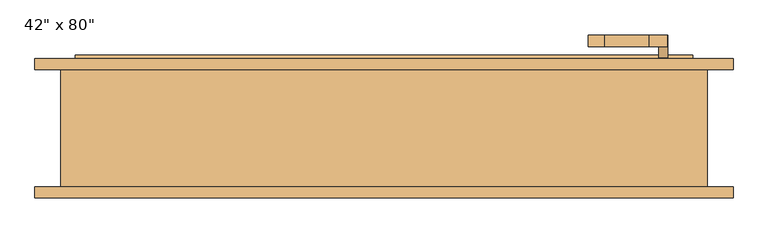
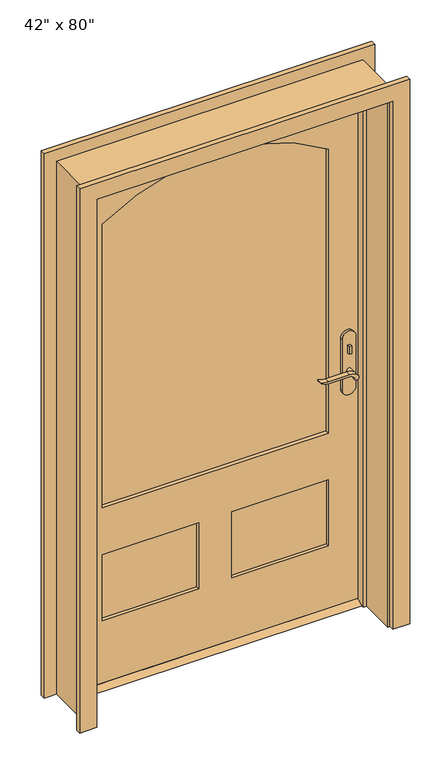
"""IFC4 building model written with IfcOpenShell, lengths in millimetres: door geometry."""

from ifc_helpers import new_model, si_unit, point, frame, frame_2d, origin, place, context, project, spatial, polyline, circle_curve, trimmed, segment, composite_curve, outline, extrude, faceted_brep, source, transform, mapped, element, save


def door_3b8e8068(model_context):
    return source(origin(), model_context, "Body", "SolidModel", [
        extrude(outline(polyline([(63.5, 12.7), (98.425, 12.7), (123.825, 0.0), (38.1, 0.0), (63.5, 12.7)])), frame((-533.4, 0.0, 0.0), z_axis=(1.0, 0.0, 0.0), x_axis=(0.0, 1.0, 0.0)), (0.0, 0.0, 1.0), 1066.8),
        extrude(outline(polyline([(487.6, 43.5), (477.6, 43.5), (477.6, 53.5), (487.6, 53.5), (487.6, 43.5)])), frame((0.0, 0.0, 981.9), z_axis=(0.0, 0.0, 1.0), x_axis=(1.0, 0.0, 0.0)), (0.0, 0.0, 1.0), 30.0),
        extrude(outline(composite_curve([segment(trimmed(circle_curve(frame_2d((996.9, 482.6)), 8.0), [point((996.9, 474.6))], [point((996.9, 490.6))], False, "CARTESIAN"), True, "CONTINUOUS"), segment(trimmed(circle_curve(frame_2d((996.9, 482.6)), 8.0), [point((996.9, 490.6))], [point((996.9, 474.6))], False, "CARTESIAN"), True, "CONTINUOUS")], self_intersect=False)), frame((0.0, 108.425, 0.0), z_axis=(0.0, 1.0, 0.0), x_axis=(0.0, 0.0, 1.0)), (0.0, 0.0, 1.0), 10.0),
        extrude(outline(composite_curve([segment(trimmed(circle_curve(frame_2d((897.1555521, 458.9324871)), 37.2832219), [point((919.0523287, 489.1081363))], [point((934.4, 457.2325667))], False, "CARTESIAN"), True, "CONTINUOUS"), segment(polyline([(934.4, 457.2325667), (934.4, 380.9564091)]), True, "CONTINUOUS"), segment(trimmed(circle_curve(frame_2d((1017.6850638, 381.0227909)), 83.2850902), [point((934.4, 380.9564091))], [point((939.4, 352.6))], True, "CARTESIAN"), True, "CONTINUOUS"), segment(polyline([(939.4, 352.6), (936.6135558, 352.6)]), True, "CONTINUOUS"), segment(trimmed(circle_curve(frame_2d((986.6709207, 384.5396612)), 59.3791355), [point((936.6135558, 352.6))], [point((927.4, 380.9564091))], False, "CARTESIAN"), True, "CONTINUOUS"), segment(polyline([(927.4, 380.9564091), (927.4, 457.2138099)]), True, "CONTINUOUS"), segment(trimmed(circle_curve(frame_2d((909.2738613, 457.2138099)), 18.1261387), [point((927.4, 457.2138099))], [point((914.4, 474.6))], True, "CARTESIAN"), True, "CONTINUOUS"), segment(trimmed(circle_curve(frame_2d((914.4, 482.6)), 8.0), [point((914.4, 474.6))], [point((919.0523287, 489.1081363))], False, "CARTESIAN"), True, "CONTINUOUS")], self_intersect=False)), frame((0.0, 3.5, 0.0), z_axis=(0.0, 1.0, 0.0), x_axis=(0.0, 0.0, 1.0)), (0.0, 0.0, 1.0), 20.0),
        extrude(outline(composite_curve([segment(trimmed(circle_curve(frame_2d((914.4, 482.6)), 8.0), [point((914.3999903, 474.6))], [point((919.0523287, 489.1081363))], False, "CARTESIAN"), True, "CONTINUOUS"), segment(trimmed(circle_curve(frame_2d((897.1555521, 458.9324871)), 37.2832219), [point((919.0523287, 489.1081363))], [point((934.4, 457.2325667))], False, "CARTESIAN"), True, "CONTINUOUS"), segment(polyline([(934.4, 457.2325667), (934.4, 380.9564091)]), True, "CONTINUOUS"), segment(trimmed(circle_curve(frame_2d((1017.6850638, 381.0227909)), 83.2850902), [point((934.4, 380.9564091))], [point((939.4, 352.6))], True, "CARTESIAN"), True, "CONTINUOUS"), segment(polyline([(939.4, 352.6), (936.6135558, 352.6)]), True, "CONTINUOUS"), segment(trimmed(circle_curve(frame_2d((986.6709207, 384.5396612)), 59.3791355), [point((936.6135558, 352.6))], [point((927.4, 380.9564091))], False, "CARTESIAN"), True, "CONTINUOUS"), segment(polyline([(927.4, 380.9564091), (927.4, 457.2138122)]), True, "CONTINUOUS"), segment(trimmed(circle_curve(frame_2d((909.2738682, 457.2138122)), 18.1261318), [point((927.4, 457.2138122))], [point((914.3999903, 474.6))], True, "CARTESIAN"), True, "CONTINUOUS")], self_intersect=False)), frame((0.0, 138.425, 0.0), z_axis=(0.0, 1.0, 0.0), x_axis=(0.0, 0.0, 1.0)), (0.0, 0.0, 1.0), 20.0),
        extrude(outline(composite_curve([segment(trimmed(circle_curve(frame_2d((914.4, 482.6)), 8.0), [point((914.4, 474.6))], [point((914.4, 490.6))], False, "CARTESIAN"), True, "CONTINUOUS"), segment(trimmed(circle_curve(frame_2d((914.4, 482.6)), 8.0), [point((914.4, 490.6))], [point((914.4, 474.6))], False, "CARTESIAN"), True, "CONTINUOUS")], self_intersect=False)), frame((0.0, 23.5, 0.0), z_axis=(0.0, 1.0, 0.0), x_axis=(0.0, 0.0, 1.0)), (0.0, 0.0, 1.0), 30.0),
        extrude(outline(composite_curve([segment(trimmed(circle_curve(frame_2d((914.4, 482.6)), 8.0), [point((914.4, 474.6))], [point((914.4, 490.6))], False, "CARTESIAN"), True, "CONTINUOUS"), segment(trimmed(circle_curve(frame_2d((914.4, 482.6)), 8.0), [point((914.4, 490.6))], [point((914.4, 474.6))], False, "CARTESIAN"), True, "CONTINUOUS")], self_intersect=False)), frame((0.0, 108.425, 0.0), z_axis=(0.0, 1.0, 0.0), x_axis=(0.0, 0.0, 1.0)), (0.0, 0.0, 1.0), 30.0),
        extrude(outline(composite_curve([segment(polyline([(844.4, 507.6), (1039.4, 507.6)]), True, "CONTINUOUS"), segment(trimmed(circle_curve(frame_2d((1039.4, 482.6)), 25.0), [point((1039.4, 507.6))], [point((1039.4, 457.6))], False, "CARTESIAN"), True, "CONTINUOUS"), segment(polyline([(1039.4, 457.6), (844.4, 457.6)]), True, "CONTINUOUS"), segment(trimmed(circle_curve(frame_2d((844.4, 482.6)), 25.0), [point((844.4, 457.6))], [point((844.4, 507.6))], False, "CARTESIAN"), True, "CONTINUOUS")], self_intersect=False)), frame((0.0, 53.5, 0.0), z_axis=(0.0, 1.0, 0.0), x_axis=(0.0, 0.0, 1.0)), (0.0, 0.0, 1.0), 10.0),
        extrude(outline(composite_curve([segment(polyline([(844.4, 507.6), (1039.4, 507.6)]), True, "CONTINUOUS"), segment(trimmed(circle_curve(frame_2d((1039.4, 482.6)), 25.0), [point((1039.4, 507.6))], [point((1039.4, 457.6))], False, "CARTESIAN"), True, "CONTINUOUS"), segment(polyline([(1039.4, 457.6), (844.4, 457.6)]), True, "CONTINUOUS"), segment(trimmed(circle_curve(frame_2d((844.4, 482.6)), 25.0), [point((844.4, 457.6))], [point((844.4, 507.6))], False, "CARTESIAN"), True, "CONTINUOUS")], self_intersect=False)), frame((0.0, 98.425, 0.0), z_axis=(0.0, 1.0, 0.0), x_axis=(0.0, 0.0, 1.0)), (0.0, 0.0, 1.0), 10.0),
        extrude(outline(polyline([(2032.0, -533.4), (12.7, -533.4), (12.7, 533.4), (2032.0, 533.4), (2032.0, -533.4)]), holes=[composite_curve([segment(polyline([(688.975, -412.75), (1784.35, -412.75)]), True, "CONTINUOUS"), segment(trimmed(circle_curve(frame_2d((1177.13125, 0.0)), 734.21875), [point((1784.35, -412.75))], [point((1784.35, 412.75))], True, "CARTESIAN"), True, "CONTINUOUS"), segment(polyline([(1784.35, 412.75), (688.975, 412.75), (688.975, -412.75)]), True, "CONTINUOUS")], self_intersect=False), polyline([(508.0, -60.325), (254.0, -60.325), (254.0, -412.75), (508.0, -412.75), (508.0, -60.325)]), polyline([(508.0, 412.75), (254.0, 412.75), (254.0, 60.325), (508.0, 60.325), (508.0, 412.75)])]), frame((0.0, 63.5, 0.0), z_axis=(0.0, 1.0, 0.0), x_axis=(0.0, 0.0, 1.0)), (0.0, 0.0, 1.0), 34.925),
        faceted_brep([(558.8, 98.425, 0.0), (558.8, -104.775, 0.0), (533.4, -104.775, 0.0), (533.4, 28.575, 0.0), (520.7, 28.575, 0.0), (520.7, 63.5, 0.0), (533.4, 63.5, 0.0), (533.4, 98.425, 0.0), (558.8, 98.425, 2057.4), (558.8, -104.775, 2057.4), (-558.8, -104.775, 2057.4), (-558.8, -104.775, 0.0), (-533.4, -104.775, 0.0), (-533.4, -104.775, 2032.0), (533.4, -104.775, 2032.0), (533.4, 28.575, 2032.0), (-533.4, 28.575, 2032.0), (-533.4, 28.575, 0.0), (-520.7, 28.575, 0.0), (-520.7, 28.575, 2019.3), (520.7, 28.575, 2019.3), (520.7, 63.5, 2019.3), (-520.7, 63.5, 2019.3), (-520.7, 63.5, 0.0), (-533.4, 63.5, 0.0), (-533.4, 63.5, 2032.0), (533.4, 63.5, 2032.0), (533.4, 98.425, 2032.0), (-533.4, 98.425, 2032.0), (-533.4, 98.425, 0.0), (-558.8, 98.425, 0.0), (-558.8, 98.425, 2057.4)], [[[0, 1, 2, 3, 4, 5, 6, 7]], [[1, 0, 8, 9]], [[2, 1, 9, 10, 11, 12, 13, 14]], [[3, 2, 14, 15]], [[4, 3, 15, 16, 17, 18, 19, 20]], [[5, 4, 20, 21]], [[6, 5, 21, 22, 23, 24, 25, 26]], [[7, 6, 26, 27]], [[0, 7, 27, 28, 29, 30, 31, 8]], [[9, 8, 31, 10]], [[15, 14, 13, 16]], [[21, 20, 19, 22]], [[27, 26, 25, 28]], [[30, 29, 24, 23, 18, 17, 12, 11]], [[10, 31, 30, 11]], [[16, 13, 12, 17]], [[22, 19, 18, 23]], [[28, 25, 24, 29]]]),
        extrude(outline(polyline([(-60.325, 75.1416667), (-412.75, 75.1416667), (-412.75, 86.7833333), (-60.325, 86.7833333), (-60.325, 75.1416667)])), frame((0.0, 0.0, 254.0), z_axis=(0.0, 0.0, 1.0), x_axis=(1.0, 0.0, 0.0)), (0.0, 0.0, 1.0), 254.0),
        extrude(outline(polyline([(412.75, 75.1416667), (60.325, 75.1416667), (60.325, 86.7833333), (412.75, 86.7833333), (412.75, 75.1416667)])), frame((0.0, 0.0, 254.0), z_axis=(0.0, 0.0, 1.0), x_axis=(1.0, 0.0, 0.0)), (0.0, 0.0, 1.0), 254.0),
        extrude(outline(composite_curve([segment(polyline([(688.975, -412.75), (688.975, 412.75), (1784.35, 412.75)]), True, "CONTINUOUS"), segment(trimmed(circle_curve(frame_2d((1177.13125, 0.0)), 734.21875), [point((1784.35, 412.75))], [point((1784.35, -412.75))], False, "CARTESIAN"), True, "CONTINUOUS"), segment(polyline([(1784.35, -412.75), (688.975, -412.75)]), True, "CONTINUOUS")], self_intersect=False)), frame((0.0, 77.47, 0.0), z_axis=(0.0, 1.0, 0.0), x_axis=(0.0, 0.0, 1.0)), (0.0, 0.0, 1.0), 6.985),
        extrude(outline(polyline([(0.0, -603.25), (0.0, -539.75), (2038.35, -539.75), (2038.35, 539.75), (0.0, 539.75), (0.0, 603.25), (2101.85, 603.25), (2101.85, -603.25), (0.0, -603.25)])), frame((0.0, -123.825, 0.0), z_axis=(0.0, 1.0, 0.0), x_axis=(0.0, 0.0, 1.0)), (0.0, 0.0, 1.0), 19.05),
        extrude(outline(polyline([(0.0, -603.25), (0.0, -539.75), (2038.35, -539.75), (2038.35, 539.75), (0.0, 539.75), (0.0, 603.25), (2101.85, 603.25), (2101.85, -603.25), (0.0, -603.25)])), frame((0.0, 98.425, 0.0), z_axis=(0.0, 1.0, 0.0), x_axis=(0.0, 0.0, 1.0)), (0.0, 0.0, 1.0), 19.05),
    ])


if __name__ == "__main__":
    model = new_model("IFC4")
    model_context = context("Model", 3, world=origin())
    ifc_project = project(units=[si_unit("LENGTHUNIT", "METRE", prefix="MILLI")], contexts=[model_context])
    site = spatial("IfcSite", under=ifc_project)
    building = spatial("IfcBuilding", under=site)
    placement = place(None, origin())
    door_shape = door_3b8e8068(model_context)
    element("IfcDoor", 1, ObjectType="42\" x 80\"", at=placement, inside=building, context=model_context, shape_type="MappedRepresentation", body=[
        mapped(door_shape, transform((0.0, 0.0, 0.0), x_axis=(1.0, 0.0, 0.0), y_axis=(0.0, 1.0, 0.0), z_axis=(0.0, 0.0, 1.0))),
    ])
    save(model, "model.ifc")

# Revit data of these elements
# Type "42\" x 80\""
#   Type Mark = "9"
#   Assembly Code = "B2030100"
#   Analytic Construction = "French door, wood frame with single glass"
#   Threshold Offset [instance default] = 0' - 0 1/2"
#   Thickness = 0' - 1 3/8"
#   Thermal Resistance (R) = 1.0696 (h·ft²·°F)/BTU
#   Swing Angle [instance default] = 90.00°
#   Stiles = 0' - 4 3/4"
#   Rough Width = 3' - 8"
#   Rough Height = 6' - 9"
#   Radius = 2' - 4 29/32"
#   Lock Rail = 0' - 7 1/8"
#   Height = 6' - 8"
#   Width = 3' - 6"
#   Heat Transfer Coefficient (U) = 0.9350 BTU/(h·ft²·°F)
#   Door Offset [instance default] = 0' - 0"
#   Bottom Rail = 0' - 9 1/2"
#   Threshold [instance default] = yes
#   Function = 1
#   Exterior Trim [instance default] = yes
#   Trim Material = Cherry
#   Threshold Material = Cherry
#   Panel Material = Cherry
#   Glazing = Glass
#   Frame Material = Cherry
#   Door Handle Material = Aluminum
#   Visual Light Transmittance = 0
#   Solar Heat Gain Coefficient = 0
#   Wall Closure = (empty or 0)
#   Construction Type = (empty or 0)
# Element 1 (IfcDoor, "42\" x 80\"")
#   Materials on its faces: "Cherry", "Aluminum", "Glass"
# Materials
#   "Cherry": class "Wood", colour RGB 226 177 128, transparency 0, Description = "Prunus Serotina", Cost = 0
#   "Glass": class "Glass", colour RGB 0 128 192, transparency 0.75, Description = "Soda Lime Glass", Cost = 0
#   "Aluminum": class "Metal", colour RGB 247 247 247, transparency 0, Description = "Aluminum 6061", Cost = 0
